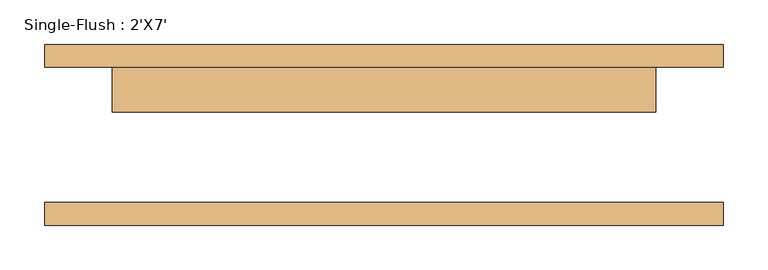
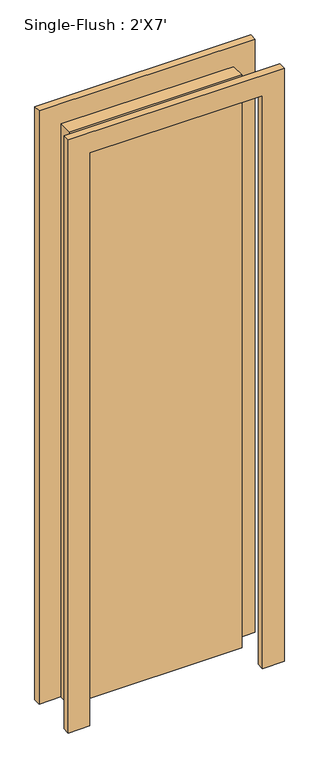
"""IFC4 building model written with IfcOpenShell, lengths in millimetres: door geometry, Single-Flush : 2'X7'."""

from ifc_helpers import new_model, si_unit, frame, origin, origin_with_axes, place, context, project, spatial, polyline, outline, extrude, source, transform, mapped, element, save


def single_flush_2_x7_9ea4ff49(model_context):
    return source(origin(), model_context, "Body", "SweptSolid", [
        extrude(outline(polyline([(2209.8, -381.0), (0.0, -381.0), (0.0, -304.8), (2133.6, -304.8), (2133.6, 304.8), (0.0, 304.8), (0.0, 381.0), (2209.8, 381.0), (2209.8, -381.0)])), frame((0.0, 76.2, 0.0), z_axis=(0.0, 1.0, 0.0), x_axis=(0.0, 0.0, 1.0)), (0.0, 0.0, 1.0), 25.4),
        extrude(outline(polyline([(2209.8, 381.0), (2209.8, -381.0), (0.0, -381.0), (0.0, -304.8), (2133.6, -304.8), (2133.6, 304.8), (0.0, 304.8), (0.0, 381.0), (2209.8, 381.0)])), frame((0.0, -101.6, 0.0), z_axis=(0.0, 1.0, 0.0), x_axis=(0.0, 0.0, 1.0)), (0.0, 0.0, 1.0), 25.4),
        extrude(outline(polyline([(304.8, 25.4), (-304.8, 25.4), (-304.8, 76.2), (304.8, 76.2), (304.8, 25.4)])), origin_with_axes(), (0.0, 0.0, 1.0), 2133.6),
    ])


if __name__ == "__main__":
    model = new_model("IFC4")
    model_context = context("Model", 3, world=origin())
    ifc_project = project(units=[si_unit("LENGTHUNIT", "METRE", prefix="MILLI")], contexts=[model_context])
    site = spatial("IfcSite", under=ifc_project)
    building = spatial("IfcBuilding", under=site)
    placement = place(None, origin())
    single_flush_2_x7_shape = single_flush_2_x7_9ea4ff49(model_context)
    element("IfcDoor", 1, ObjectType="Single-Flush : 2'X7'", at=placement, inside=building, context=model_context, shape_type="MappedRepresentation", body=[
        mapped(single_flush_2_x7_shape, transform((0.0, 0.0, 0.0), x_axis=(1.0, 0.0, 0.0), y_axis=(0.0, 1.0, 0.0), z_axis=(0.0, 0.0, 1.0))),
    ])
    save(model, "model.ifc")

# Revit data of these elements
# Type "Single-Flush : 2'X7'"
#   Type Mark = "12"
#   Construction Type Id = "MDOOR"
#   Assembly Code = "C1020"
#   Analytic Construction = "Metal"
#   Thickness = 0' - 2"
#   Heat Transfer Coefficient (U) = 0.651978 BTU/(h·ft²·°F)
#   Height = 7' - 0"
#   Trim Projection Ext = 0' - 1"
#   Trim Projection Int = 0' - 1"
#   Trim Width = 0' - 3"
#   Width = 2' - 0"
#   Define Thermal Properties by = 1
#   Door Material = Door - Panel
#   Frame Material = Door - Frame
#   Visual Light Transmittance = 0
#   Solar Heat Gain Coefficient = 0
#   Function = (empty or 0)
#   Wall Closure = (empty or 0)
# Element 1 (IfcDoor, "Single-Flush : 2'X7'")
#   Materials on its faces: "Door - Frame", "Door - Panel"
# Materials
#   "Door - Panel": class "Wood", colour RGB 210 159 95, transparency 0, Cost = 0
#   "Door - Frame": colour RGB 118 70 51, transparency 0, Cost = 0
